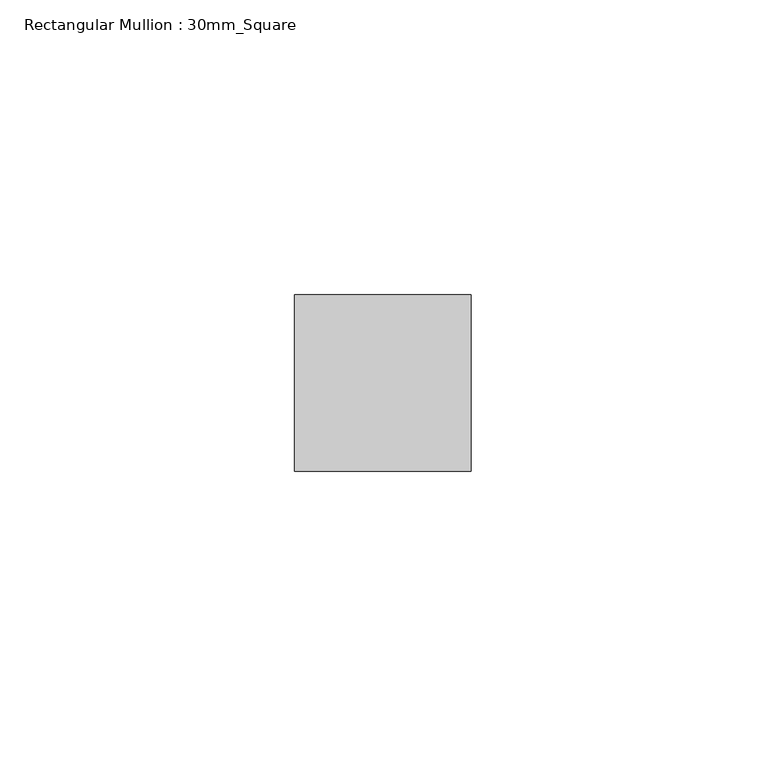
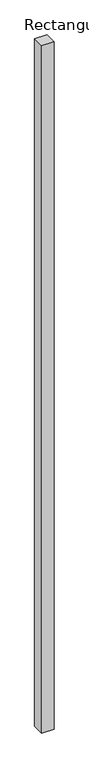
"""IFC4 building model written with IfcOpenShell, lengths in millimetres: member geometry, Rectangular Mullion : 30mm_Square."""

from ifc_helpers import new_model, si_unit, frame, origin, place, context, project, spatial, polyline, outline, extrude, source, transform, mapped, element, save


def rectangular_mullion_30mm_square_5c6859bd(model_context):
    return source(origin(), model_context, "Body", "SweptSolid", [
        extrude(outline(polyline([(0.0, 15.0), (0.0, -15.0), (-30.0, -15.0), (-30.0, 15.0), (0.0, 15.0)])), frame((0.0, 0.0, -1782.0004658), z_axis=(0.0, 0.0, 1.0), x_axis=(1.0, 0.0, 0.0)), (0.0, 0.0, 1.0), 1782.0004658),
    ])


if __name__ == "__main__":
    model = new_model("IFC4")
    model_context = context("Model", 3, world=origin())
    ifc_project = project(units=[si_unit("LENGTHUNIT", "METRE", prefix="MILLI")], contexts=[model_context])
    site = spatial("IfcSite", under=ifc_project)
    building = spatial("IfcBuilding", under=site)
    placement = place(None, origin())
    rectangular_mullion_30mm_square_shape = rectangular_mullion_30mm_square_5c6859bd(model_context)
    element("IfcMember", 1, ObjectType="Rectangular Mullion : 30mm_Square", at=placement, inside=building, context=model_context, shape_type="MappedRepresentation", body=[
        mapped(rectangular_mullion_30mm_square_shape, transform((0.0, 0.0, 0.0), x_axis=(1.0, 0.0, 0.0), y_axis=(0.0, 1.0, 0.0), z_axis=(0.0, 0.0, 1.0))),
    ])
    save(model, "model.ifc")

# Revit data of these elements
# Type "Rectangular Mullion : 30mm_Square"
#   Keynote = "H11"
#   built-in parameter 1007304 = 0.0984252 (stored number, unit not read)
#   built-in parameter 1007301 = 0.0492126 (stored number, unit not read)
#   built-in parameter 1007300 = 0.0492126 (stored number, unit not read)
# Element 1 (IfcMember, "Rectangular Mullion : 30mm_Square")
#   Materials on its faces: "Aluminium"
# Materials
#   "Aluminium": class "Metal", colour RGB 247 247 247, transparency 0, Description = "Aluminium 6061", Cost = 0
